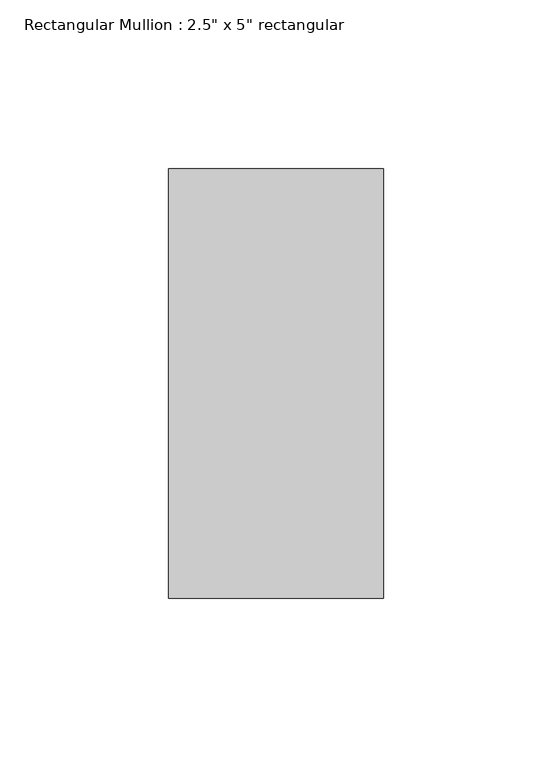
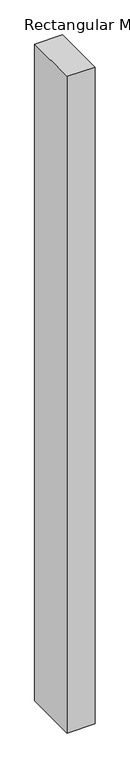
"""IFC4 building model written with IfcOpenShell, lengths in millimetres: member geometry."""

from ifc_helpers import new_model, si_unit, frame, origin, place, context, project, spatial, polyline, outline, extrude, source, transform, mapped, element, save


def member_591cd9a7(model_context):
    return source(origin(), model_context, "Body", "SweptSolid", [
        extrude(outline(polyline([(31.75, 63.5), (31.75, -63.5), (-31.75, -63.5), (-31.75, 63.5), (31.75, 63.5)])), frame((0.0, 0.0, -1574.8), z_axis=(0.0, 0.0, 1.0), x_axis=(1.0, 0.0, 0.0)), (0.0, 0.0, 1.0), 1574.8),
    ])


if __name__ == "__main__":
    model = new_model("IFC4")
    model_context = context("Model", 3, world=origin())
    ifc_project = project(units=[si_unit("LENGTHUNIT", "METRE", prefix="MILLI")], contexts=[model_context])
    site = spatial("IfcSite", under=ifc_project)
    building = spatial("IfcBuilding", under=site)
    placement = place(None, origin())
    member_shape = member_591cd9a7(model_context)
    element("IfcMember", 1, ObjectType="Rectangular Mullion : 2.5\" x 5\" rectangular", at=placement, inside=building, context=model_context, shape_type="MappedRepresentation", body=[
        mapped(member_shape, transform((0.0, 0.0, 0.0), x_axis=(1.0, 0.0, 0.0), y_axis=(0.0, 1.0, 0.0), z_axis=(0.0, 0.0, 1.0))),
    ])
    save(model, "model.ifc")

# Revit data of these elements
# Type "Rectangular Mullion : 2.5\" x 5\" rectangular"
#   built-in parameter 1007304 = 0.416667 (stored number, unit not read)
#   built-in parameter 1007301 = 0.104167 (stored number, unit not read)
#   built-in parameter 1007300 = 0.104167 (stored number, unit not read)
# Element 1 (IfcMember, "Rectangular Mullion : 2.5\" x 5\" rectangular")
#   Materials on its faces: "Aluminum"
# Materials
#   "Aluminum": class "Metal", colour RGB 247 247 247, transparency 0, Description = "Aluminum 6061", Cost = 0
